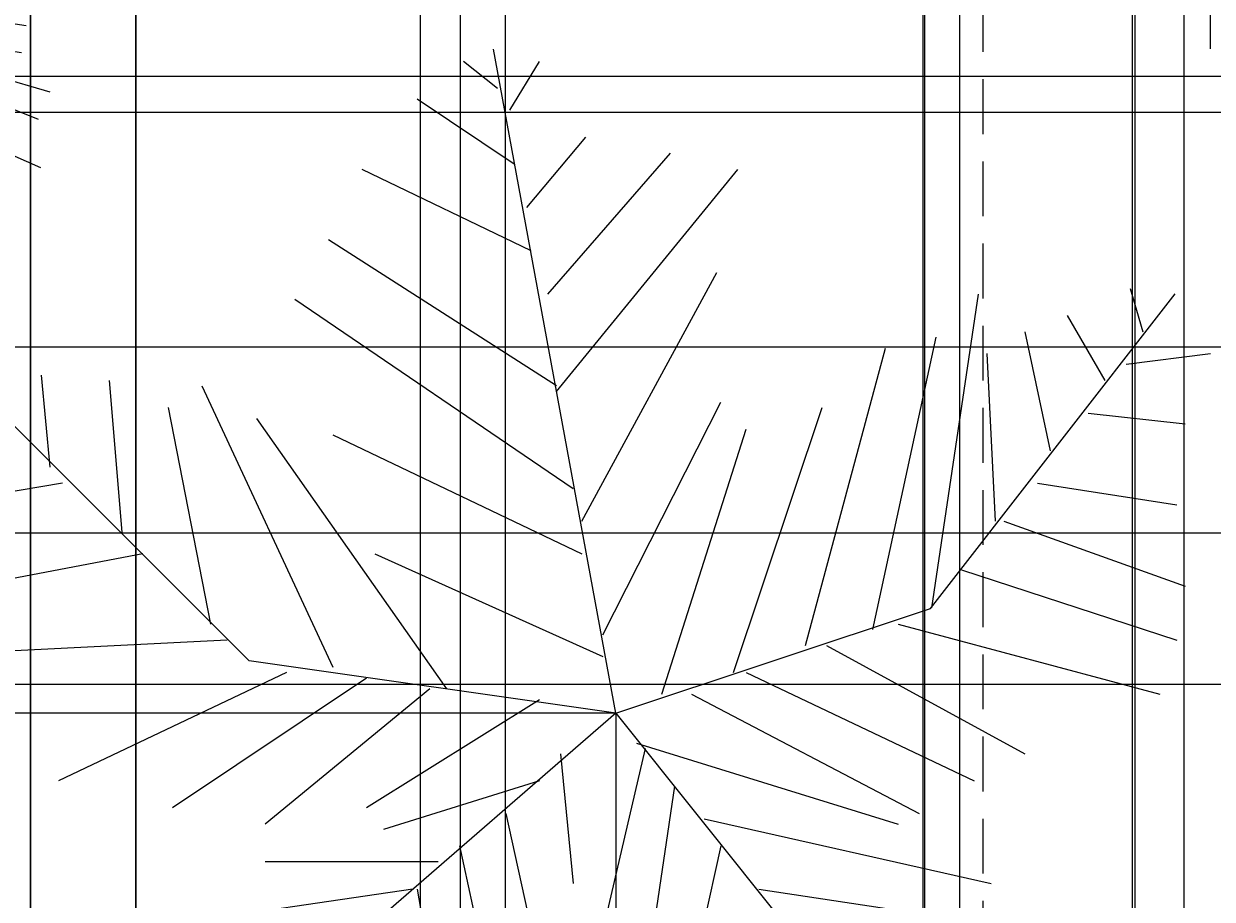
# Model space of a CAD drawing. Units: inches. Extents: x 818 to 1898, y 976 to 2364.
# Tile 13 of 96: x 1071 to 1207, y 1773 to 1873. Entities that reach past the tile are written whole.
import ezdxf

# ---------------------------------------------------------------- set-up
doc = ezdxf.new("R2010")
doc.units = ezdxf.units.IN
doc.header["$LTSCALE"] = 5
doc.header["$MEASUREMENT"] = 0
doc.linetypes.add('HIDDEN', pattern=[0.375, 0.25, -0.125])
for name, color, linetype, lineweight in [('A-ANNO-DIMS', 2, 'Continuous', 18), ('A-FLOR-OVHD', 8, 'HIDDEN', 13), ('L-PLNT-BEDS', 94, 'Continuous', 18)]:
    doc.layers.add(name, color=color, linetype=linetype, lineweight=lineweight)
doc.layers.add('L-PLNT', color=116, linetype='Continuous', lineweight=13, true_color=0x136734)
doc.styles.get("Standard").update_dxf_attribs({"font": 'arial.ttf'})
doc.dimstyles.get("Standard").update_dxf_attribs({"dimtxt": 0.18, "dimasz": 0.18, "dimexe": 0.18, "dimexo": 0.0625, "dimgap": 0.09, "dimtad": 0, "dimtih": 1, "dimtoh": 1, "dimdec": 4, "dimzin": 0, "dimdsep": 46, "dimtxsty": 'Standard', "dimcen": 0.09, "dimadec": 0, "dimazin": 0, "dimtfac": 1, "dimtdec": 4, "dimtofl": 0, "dimtmove": 0, "dimatfit": 3, "dimfxl": 1, "dimtolj": 1, "dimtzin": 0, "dimarcsym": 0})

# ---------------------------------------------------------------- blocks, each defined once
blk = doc.blocks.new('PALM-BORDER')
for p, q in [((41.53, 39.05), (33.72, 81.45)), ((33.95, 78.95), (31.8, 80.68)), ((34.76, 77.57), (36.65, 80.68)), ((35.03, 74.11), (28.83, 78.26)), ((35.84, 71.35), (39.61, 75.84)), ((37.18, 65.82), (45, 74.8)), ((36.11, 68.59), (25.33, 73.77)), ((37.72, 59.6), (49.31, 73.77)), ((37.72, 59.95), (23.17, 69.28)), ((39.34, 51.31), (47.96, 67.2)), ((38.8, 53.39), (21.02, 65.48)), ((61.61, 45.75), (77.23, 65.83)), ((61.71, 45.79), (64.67, 65.82)), ((74.37, 66.17), (75.18, 63.4)), ((70.33, 64.44), (72.75, 60.3)), ((53.62, 43.37), (58.74, 62.37)), ((57.93, 44.41), (61.97, 63.06)), ((67.63, 63.4), (69.25, 55.81)), ((65.21, 62.02), (65.75, 51.31)), ((74.1, 61.33), (79.49, 62.02)), ((5.39, 54.77), (4.85, 60.64)), ((9.16, 60.3), (9.97, 50.62)), ((15.09, 59.95), (23.44, 41.99)), ((12.93, 58.57), (15.63, 44.75)), ((40.69, 44.06), (48.23, 58.91)), ((49.04, 41.64), (54.7, 58.57)), ((18.1, 42.4), (2.48, 58.02)), ((30.72, 40.61), (18.59, 57.88)), ((44.46, 40.26), (49.85, 57.19)), ((71.68, 58.22), (77.87, 57.53)), ((23.44, 56.84), (39.34, 49.24)), ((6.2, 53.73), (0, 52.7)), ((68.44, 53.73), (77.33, 52.35)), ((66.29, 51.31), (77.87, 47.17)), ((11.32, 49.24), (0.54, 47.17)), ((26.14, 49.24), (40.69, 42.68)), ((63.59, 48.21), (77.33, 43.71)), ((41.53, 39.05), (61.61, 45.75)), ((59.55, 44.75), (76.26, 40.26)), ((16.71, 43.71), (2.69, 43.02)), ((41.53, 39.05), (18.1, 42.4)), ((54.97, 43.37), (67.63, 36.46)), ((20.48, 41.64), (5.93, 34.73)), ((25.6, 41.3), (13.2, 33.01)), ((49.85, 41.64), (64.4, 34.73)), ((29.64, 40.61), (19.13, 31.97)), ((36.65, 39.91), (25.6, 33.01)), ((46.35, 40.26), (60.9, 32.66)), ((41.53, 39.05), (24.79, 24.55)), ((41.53, 39.05), (54.92, 22.32)), ((43.38, 36.81), (40.42, 24.02)), ((42.84, 37.15), (59.55, 31.97)), ((37.99, 36.46), (38.8, 28.17)), ((36.65, 34.73), (26.68, 31.62)), ((45.27, 34.39), (43.11, 19.88)), ((34.49, 32.66), (36.92, 21.61)), ((47.15, 32.32), (65.48, 28.17)), ((31.53, 30.59), (35.03, 14.7)), ((48.23, 30.59), (44.19, 12.28)), ((30.18, 29.55), (19.13, 29.55)), ((28.56, 27.82), (9.7, 25.06)), ((28.83, 27.82), (32.07, 9.17)), ((50.66, 27.82), (68.98, 25.06)), ((52, 26.44), (46.35, 9.17)), ((24.79, 24.55), (13.63, 5.58)), ((26.14, 25.41), (28.29, 6.06)), ((53.62, 24.37), (68.44, 21.95)), ((23.44, 22.99), (9.97, 22.64)), ((54.97, 22.3), (47.69, 5.02)), ((54.92, 22.32), (61.61, 0)), ((55.24, 22.3), (71.68, 17.46)), ((22.9, 21.26), (24.52, 5.37)), ((21.56, 19.53), (11.59, 19.88)), ((55.78, 20.22), (70.33, 14.35)), ((20.48, 17.46), (9.7, 15.73)), ((56.59, 16.42), (53.35, 5.72)), ((19.94, 16.08), (20.75, 6.41)), ((18.59, 13.66), (9.97, 12.62)), ((57.39, 14.7), (70.6, 8.83)), ((17.24, 11.59), (17.78, 6.06)), ((58.47, 10.9), (56.05, 2.95)), ((15.9, 9.52), (11.05, 7.44)), ((58.47, 10.55), (67.09, 5.72)), ((59.82, 6.75), (64.4, 3.64)), ((59.82, 5.02), (58.74, 1.22)), ((61.44, 1.92), (62.51, 1.22))]:
    blk.add_line(p, q)
blk = doc.blocks.new('PALM-DECK')
for p, q in [((74.19, 69.77), (60.24, 145.52)), ((60.66, 141.05), (56.81, 144.14)), ((62.1, 138.58), (65.47, 144.14)), ((62.58, 132.41), (51.51, 139.82)), ((64.03, 127.47), (70.77, 135.5)), ((66.43, 117.6), (80.4, 133.65)), ((64.51, 122.54), (45.25, 131.79)), ((67.4, 106.49), (88.1, 131.79)), ((67.4, 107.11), (41.4, 123.77)), ((70.29, 91.68), (85.69, 120.07)), ((132.87, 118.22), (134.31, 113.28)), ((69.32, 95.38), (37.55, 116.98)), ((110.08, 81.73), (137.98, 117.61)), ((110.24, 81.8), (115.54, 117.6)), ((125.65, 115.13), (129.98, 107.72)), ((103.5, 79.33), (110.72, 112.66)), ((120.83, 113.28), (123.72, 99.7)), ((95.8, 77.48), (104.95, 111.43)), ((116.5, 110.81), (117.47, 91.68)), ((132.39, 109.58), (142.02, 110.81)), ((9.63, 97.85), (8.67, 108.34)), ((16.37, 107.72), (17.81, 90.44)), ((26.96, 107.11), (41.88, 75.01)), ((23.11, 104.64), (27.92, 79.95)), ((72.69, 78.72), (86.17, 105.26)), ((87.62, 74.4), (97.73, 104.64)), ((32.33, 75.75), (4.43, 103.66)), ((54.88, 72.55), (33.22, 103.4)), ((128.06, 104.02), (139.13, 102.79)), ((79.43, 71.93), (89.06, 102.17)), ((41.88, 101.55), (70.29, 87.97)), ((11.07, 96), (0, 94.15)), ((122.28, 96), (138.16, 93.53)), ((118.43, 91.68), (139.13, 84.27)), ((20.22, 87.97), (0.96, 84.27)), ((46.7, 87.97), (72.69, 76.25)), ((113.61, 86.12), (138.16, 78.1)), ((74.19, 69.77), (110.08, 81.73)), ((106.39, 79.95), (136.24, 71.93)), ((29.85, 78.1), (4.81, 76.87)), ((98.21, 77.48), (120.83, 65.14)), ((74.19, 69.77), (32.33, 75.75)), ((36.59, 74.4), (10.59, 62.05)), ((45.73, 73.78), (23.59, 58.97)), ((89.06, 74.4), (115.06, 62.05)), ((52.96, 72.55), (34.18, 57.12)), ((82.8, 71.93), (108.8, 58.35)), ((65.47, 71.31), (45.73, 58.97)), ((74.19, 69.77), (44.29, 43.85)), ((74.19, 69.77), (98.11, 39.87)), ((67.88, 65.14), (69.32, 50.33)), ((77.51, 65.76), (72.21, 42.92)), ((76.54, 66.37), (106.39, 57.12)), ((65.47, 62.05), (47.66, 56.5)), ((80.88, 61.44), (77.03, 35.52)), ((61.62, 58.35), (65.95, 38.6)), ((84.25, 57.73), (116.98, 50.33)), ((56.33, 54.65), (62.58, 26.26)), ((86.17, 54.65), (78.95, 21.94)), ((53.92, 52.8), (34.18, 52.8)), ((51.03, 49.71), (17.33, 44.77)), ((51.51, 49.71), (57.29, 16.38)), ((90.51, 49.71), (123.24, 44.77))]:
    blk.add_line(p, q)
blk = doc.blocks.new('*D29')
at = {"layer": 'A-ANNO-DIMS', "color": 0, "lineweight": -2, "ltscale": 5, "transparency": 16777216}
for p, q in [((1064.31, 1870.24), (1064.31, 1892.19)), ((1064.49, 1892.01), (1134.73, 1892.01)), ((1206.15, 1892.01), (1135.91, 1892.01)), ((1206.33, 1870.24), (1206.33, 1892.19))]:
    blk.add_line(p, q, dxfattribs=at)
at = {"layer": 'A-ANNO-DIMS', "color": 0, "ltscale": 5, "transparency": 16777216}
for points in [[(1064.49, 1892.04), (1064.49, 1891.98), (1064.31, 1892.01)], [(1206.15, 1892.04), (1206.15, 1891.98), (1206.33, 1892.01)]]:
    blk.add_solid(points, dxfattribs=at)
at = {"layer": 'Defpoints', "color": 0, "ltscale": 5, "transparency": 16777216}
for p in [(1206.33, 1892.01), (1064.31, 1870.18), (1206.33, 1870.18)]:
    blk.add_point(p, dxfattribs=at)
at = {"layer": 'A-ANNO-DIMS', "color": 0, "ltscale": 5, "transparency": 16777216, "insert": (1135.32, 1892.01), "char_height": 0.18, "attachment_point": 5}
blk.add_mtext('\\A1;142 TYP.', dxfattribs=at)
blk = doc.blocks.new('*D59')
at = {"layer": 'A-ANNO-DIMS', "color": 0, "lineweight": -2, "ltscale": 5, "transparency": 16777216}
for p, q in [((1251.64, 2300.39), (818.03, 2300.39)), ((818.21, 2300.21), (818.21, 1669.95)), ((818.21, 1039.32), (818.21, 1669.59)), ((896.05, 1039.14), (818.03, 1039.14))]:
    blk.add_line(p, q, dxfattribs=at)
at = {"layer": 'A-ANNO-DIMS', "color": 0, "ltscale": 5, "transparency": 16777216}
for points in [[(818.18, 2300.21), (818.24, 2300.21), (818.21, 2300.39)], [(818.18, 1039.32), (818.24, 1039.32), (818.21, 1039.14)]]:
    blk.add_solid(points, dxfattribs=at)
at = {"layer": 'Defpoints', "color": 0, "ltscale": 5, "transparency": 16777216}
for p in [(818.21, 2300.39), (1251.71, 2300.39), (896.11, 1039.14)]:
    blk.add_point(p, dxfattribs=at)
at = {"layer": 'A-ANNO-DIMS', "color": 0, "ltscale": 5, "transparency": 16777216, "insert": (818.21, 1669.77), "char_height": 0.18, "attachment_point": 5}
blk.add_mtext('\\A1;1261.2', dxfattribs=at)
blk = doc.blocks.new('*D61')
at = {"layer": 'A-ANNO-DIMS', "color": 0, "lineweight": -2, "ltscale": 5, "transparency": 16777216}
for p, q in [((1071.73, 1203.03), (1071.73, 2363.87)), ((1071.91, 2363.69), (1250.94, 2363.69)), ((1430.55, 2363.69), (1251.51, 2363.69)), ((1430.73, 1203.03), (1430.73, 2363.87))]:
    blk.add_line(p, q, dxfattribs=at)
at = {"layer": 'A-ANNO-DIMS', "color": 0, "ltscale": 5, "transparency": 16777216}
for points in [[(1071.91, 2363.72), (1071.91, 2363.66), (1071.73, 2363.69)], [(1430.55, 2363.72), (1430.55, 2363.66), (1430.73, 2363.69)]]:
    blk.add_solid(points, dxfattribs=at)
at = {"layer": 'Defpoints', "color": 0, "ltscale": 5, "transparency": 16777216}
for p in [(1430.73, 2363.69), (1071.73, 1202.96), (1430.73, 1202.96)]:
    blk.add_point(p, dxfattribs=at)
at = {"layer": 'A-ANNO-DIMS', "color": 0, "ltscale": 5, "transparency": 16777216, "insert": (1251.23, 2363.69), "char_height": 0.18, "attachment_point": 5}
blk.add_mtext('\\A1;359', dxfattribs=at)
blk = doc.blocks.new('*D64')
at = {"layer": 'A-ANNO-DIMS', "color": 0, "lineweight": -2, "ltscale": 5, "transparency": 16777216}
for p, q in [((1197.73, 1501.14), (1197.73, 2363.87)), ((1197.91, 2363.69), (1313.93, 2363.69)), ((1430.55, 2363.69), (1314.52, 2363.69)), ((1430.73, 1501.14), (1430.73, 2363.87))]:
    blk.add_line(p, q, dxfattribs=at)
at = {"layer": 'A-ANNO-DIMS', "color": 0, "ltscale": 5, "transparency": 16777216}
for points in [[(1197.91, 2363.72), (1197.91, 2363.66), (1197.73, 2363.69)], [(1430.55, 2363.72), (1430.55, 2363.66), (1430.73, 2363.69)]]:
    blk.add_solid(points, dxfattribs=at)
at = {"layer": 'Defpoints', "color": 0, "ltscale": 5, "transparency": 16777216}
for p in [(1430.73, 2363.69), (1197.73, 1501.08), (1430.73, 1501.08)]:
    blk.add_point(p, dxfattribs=at)
at = {"layer": 'A-ANNO-DIMS', "color": 0, "ltscale": 5, "transparency": 16777216, "insert": (1314.23, 2363.69), "char_height": 0.18, "attachment_point": 5}
blk.add_mtext('\\A1;233', dxfattribs=at)
blk = doc.blocks.new('*D79')
at = {"layer": 'A-ANNO-DIMS', "color": 0, "lineweight": -2, "ltscale": 5, "transparency": 16777216}
for p, q in [((992.73, 1203.03), (992.73, 2363.87)), ((992.91, 2363.69), (1032.01, 2363.69)), ((1071.55, 2363.69), (1032.44, 2363.69)), ((1071.73, 1203.03), (1071.73, 2363.87))]:
    blk.add_line(p, q, dxfattribs=at)
at = {"layer": 'A-ANNO-DIMS', "color": 0, "ltscale": 5, "transparency": 16777216}
for points in [[(992.91, 2363.72), (992.91, 2363.66), (992.73, 2363.69)], [(1071.55, 2363.72), (1071.55, 2363.66), (1071.73, 2363.69)]]:
    blk.add_solid(points, dxfattribs=at)
at = {"layer": 'Defpoints', "color": 0, "ltscale": 5, "transparency": 16777216}
for p in [(1071.73, 2363.69), (992.73, 1202.96), (1071.73, 1202.96)]:
    blk.add_point(p, dxfattribs=at)
at = {"layer": 'A-ANNO-DIMS', "color": 0, "ltscale": 5, "transparency": 16777216, "insert": (1032.23, 2363.69), "char_height": 0.18, "attachment_point": 5}
blk.add_mtext('\\A1;79', dxfattribs=at)
blk = doc.blocks.new('*D82')
at = {"layer": 'A-ANNO-DIMS', "color": 0, "lineweight": -2, "ltscale": 5, "transparency": 16777216}
for p, q in [((1083.73, 1501.14), (1083.73, 2363.87)), ((1083.91, 2363.69), (1140.45, 2363.69)), ((1197.55, 2363.69), (1141.01, 2363.69)), ((1197.73, 1501.14), (1197.73, 2363.87))]:
    blk.add_line(p, q, dxfattribs=at)
at = {"layer": 'A-ANNO-DIMS', "color": 0, "ltscale": 5, "transparency": 16777216}
for points in [[(1083.91, 2363.72), (1083.91, 2363.66), (1083.73, 2363.69)], [(1197.55, 2363.72), (1197.55, 2363.66), (1197.73, 2363.69)]]:
    blk.add_solid(points, dxfattribs=at)
at = {"layer": 'Defpoints', "color": 0, "ltscale": 5, "transparency": 16777216}
for p in [(1197.73, 2363.69), (1083.73, 1501.08), (1197.73, 1501.08)]:
    blk.add_point(p, dxfattribs=at)
at = {"layer": 'A-ANNO-DIMS', "color": 0, "ltscale": 5, "transparency": 16777216, "insert": (1140.73, 2363.69), "char_height": 0.18, "attachment_point": 5}
blk.add_mtext('\\A1;114', dxfattribs=at)
blk = doc.blocks.new('*D83')
at = {"layer": 'A-ANNO-DIMS', "color": 0, "lineweight": -2, "ltscale": 5, "transparency": 16777216}
for p, q in [((1197.73, 1700.14), (1197.73, 2363.87)), ((1197.91, 2363.69), (1228.02, 2363.69)), ((1258.55, 2363.69), (1228.43, 2363.69)), ((1258.73, 1700.14), (1258.73, 2363.87))]:
    blk.add_line(p, q, dxfattribs=at)
at = {"layer": 'A-ANNO-DIMS', "color": 0, "ltscale": 5, "transparency": 16777216}
for points in [[(1197.91, 2363.72), (1197.91, 2363.66), (1197.73, 2363.69)], [(1258.55, 2363.72), (1258.55, 2363.66), (1258.73, 2363.69)]]:
    blk.add_solid(points, dxfattribs=at)
at = {"layer": 'Defpoints', "color": 0, "ltscale": 5, "transparency": 16777216}
for p in [(1258.73, 2363.69), (1197.73, 1700.08), (1258.73, 1700.08)]:
    blk.add_point(p, dxfattribs=at)
at = {"layer": 'A-ANNO-DIMS', "color": 0, "ltscale": 5, "transparency": 16777216, "insert": (1228.23, 2363.69), "char_height": 0.18, "attachment_point": 5}
blk.add_mtext('\\A1;61', dxfattribs=at)
blk = doc.blocks.new('*D93')
at = {"layer": 'A-ANNO-DIMS', "color": 0, "lineweight": -2, "ltscale": 5, "transparency": 16777216}
for p, q in [((1068.34, 1071.12), (1068.34, 2363.87)), ((1068.52, 2363.69), (1094.16, 2363.69)), ((1120.58, 2363.69), (1094.94, 2363.69)), ((1120.76, 1071.12), (1120.76, 2363.87))]:
    blk.add_line(p, q, dxfattribs=at)
at = {"layer": 'A-ANNO-DIMS', "color": 0, "ltscale": 5, "transparency": 16777216}
for points in [[(1068.52, 2363.72), (1068.52, 2363.66), (1068.34, 2363.69)], [(1120.58, 2363.72), (1120.58, 2363.66), (1120.76, 2363.69)]]:
    blk.add_solid(points, dxfattribs=at)
at = {"layer": 'Defpoints', "color": 0, "ltscale": 5, "transparency": 16777216}
for p in [(1120.76, 2363.69), (1068.34, 1071.06), (1120.76, 1071.06)]:
    blk.add_point(p, dxfattribs=at)
at = {"layer": 'A-ANNO-DIMS', "color": 0, "ltscale": 5, "transparency": 16777216, "insert": (1094.55, 2363.69), "char_height": 0.18, "attachment_point": 5}
blk.add_mtext('\\A1;52.42', dxfattribs=at)
blk = doc.blocks.new('*D94')
at = {"layer": 'A-ANNO-DIMS', "color": 0, "lineweight": -2, "ltscale": 5, "transparency": 16777216}
for p, q in [((1120.76, 1071.12), (1120.76, 2363.87)), ((1120.94, 2363.69), (1146.76, 2363.69)), ((1173.36, 2363.69), (1147.55, 2363.69)), ((1173.54, 1071.12), (1173.54, 2363.87))]:
    blk.add_line(p, q, dxfattribs=at)
at = {"layer": 'A-ANNO-DIMS', "color": 0, "ltscale": 5, "transparency": 16777216}
for points in [[(1120.94, 2363.72), (1120.94, 2363.66), (1120.76, 2363.69)], [(1173.36, 2363.72), (1173.36, 2363.66), (1173.54, 2363.69)]]:
    blk.add_solid(points, dxfattribs=at)
at = {"layer": 'Defpoints', "color": 0, "ltscale": 5, "transparency": 16777216}
for p in [(1173.54, 2363.69), (1120.76, 1071.06), (1173.54, 1071.06)]:
    blk.add_point(p, dxfattribs=at)
at = {"layer": 'A-ANNO-DIMS', "color": 0, "ltscale": 5, "transparency": 16777216, "insert": (1147.15, 2363.69), "char_height": 0.18, "attachment_point": 5}
blk.add_mtext('\\A1;52.78', dxfattribs=at)
blk = doc.blocks.new('*D95')
at = {"layer": 'A-ANNO-DIMS', "color": 0, "lineweight": -2, "ltscale": 5, "transparency": 16777216}
for p, q in [((1173.54, 1071.12), (1173.54, 2363.87)), ((1173.72, 2363.69), (1201.29, 2363.69)), ((1229.47, 2363.69), (1201.9, 2363.69)), ((1229.65, 1071.12), (1229.65, 2363.87))]:
    blk.add_line(p, q, dxfattribs=at)
at = {"layer": 'A-ANNO-DIMS', "color": 0, "ltscale": 5, "transparency": 16777216}
for points in [[(1173.72, 2363.72), (1173.72, 2363.66), (1173.54, 2363.69)], [(1229.47, 2363.72), (1229.47, 2363.66), (1229.65, 2363.69)]]:
    blk.add_solid(points, dxfattribs=at)
at = {"layer": 'Defpoints', "color": 0, "ltscale": 5, "transparency": 16777216}
for p in [(1229.65, 2363.69), (1173.54, 1071.06), (1229.65, 1071.06)]:
    blk.add_point(p, dxfattribs=at)
at = {"layer": 'A-ANNO-DIMS', "color": 0, "ltscale": 5, "transparency": 16777216, "insert": (1201.59, 2363.69), "char_height": 0.18, "attachment_point": 5}
blk.add_mtext('\\A1;56.1', dxfattribs=at)
blk = doc.blocks.new('*D109')
at = {"layer": 'A-ANNO-DIMS', "color": 0, "lineweight": -2, "ltscale": 5, "transparency": 16777216}
for p, q in [((1125.92, 1410.12), (1125.92, 2363.87)), ((1126.1, 2363.69), (1164.25, 2363.69)), ((1203.15, 2363.69), (1165, 2363.69)), ((1203.33, 1409.91), (1203.33, 2363.87))]:
    blk.add_line(p, q, dxfattribs=at)
at = {"layer": 'A-ANNO-DIMS', "color": 0, "ltscale": 5, "transparency": 16777216}
for points in [[(1126.1, 2363.72), (1126.1, 2363.66), (1125.92, 2363.69)], [(1203.15, 2363.72), (1203.15, 2363.66), (1203.33, 2363.69)]]:
    blk.add_solid(points, dxfattribs=at)
at = {"layer": 'Defpoints', "color": 0, "ltscale": 5, "transparency": 16777216}
for p in [(1203.33, 2363.69), (1125.92, 1410.05), (1203.33, 1409.85)]:
    blk.add_point(p, dxfattribs=at)
at = {"layer": 'A-ANNO-DIMS', "color": 0, "ltscale": 5, "transparency": 16777216, "insert": (1164.62, 2363.69), "char_height": 0.18, "attachment_point": 5}
blk.add_mtext('\\A1;77.41', dxfattribs=at)
blk = doc.blocks.new('*D120')
at = {"layer": 'A-ANNO-DIMS', "color": 0, "lineweight": -2, "ltscale": 5, "transparency": 16777216}
for p, q in [((1766.29, 1797.72), (818.03, 1797.72)), ((818.21, 1797.54), (818.21, 1757.53)), ((818.21, 1717.17), (818.21, 1757.17)), ((1766.29, 1716.99), (818.03, 1716.99))]:
    blk.add_line(p, q, dxfattribs=at)
at = {"layer": 'A-ANNO-DIMS', "color": 0, "ltscale": 5, "transparency": 16777216}
for points in [[(818.18, 1797.54), (818.24, 1797.54), (818.21, 1797.72)], [(818.18, 1717.17), (818.24, 1717.17), (818.21, 1716.99)]]:
    blk.add_solid(points, dxfattribs=at)
at = {"layer": 'Defpoints', "color": 0, "ltscale": 5, "transparency": 16777216}
for p in [(818.21, 1797.72), (1766.35, 1797.72), (1766.35, 1716.99)]:
    blk.add_point(p, dxfattribs=at)
at = {"layer": 'A-ANNO-DIMS', "color": 0, "ltscale": 5, "transparency": 16777216, "insert": (818.21, 1757.35), "char_height": 0.18, "attachment_point": 5}
blk.add_mtext('\\A1;80.73', dxfattribs=at)
blk = doc.blocks.new('*D121')
at = {"layer": 'A-ANNO-DIMS', "color": 0, "lineweight": -2, "ltscale": 5, "transparency": 16777216}
for p, q in [((1766.29, 1884.2), (818.03, 1884.2)), ((818.21, 1884.02), (818.21, 1841.14)), ((818.21, 1797.9), (818.21, 1840.78)), ((1766.29, 1797.72), (818.03, 1797.72))]:
    blk.add_line(p, q, dxfattribs=at)
at = {"layer": 'A-ANNO-DIMS', "color": 0, "ltscale": 5, "transparency": 16777216}
for points in [[(818.18, 1884.02), (818.24, 1884.02), (818.21, 1884.2)], [(818.18, 1797.9), (818.24, 1797.9), (818.21, 1797.72)]]:
    blk.add_solid(points, dxfattribs=at)
at = {"layer": 'Defpoints', "color": 0, "ltscale": 5, "transparency": 16777216}
for p in [(818.21, 1884.2), (1766.35, 1884.2), (1766.35, 1797.72)]:
    blk.add_point(p, dxfattribs=at)
at = {"layer": 'A-ANNO-DIMS', "color": 0, "ltscale": 5, "transparency": 16777216, "insert": (818.21, 1840.96), "char_height": 0.18, "attachment_point": 5}
blk.add_mtext('\\A1;86.49', dxfattribs=at)
blk = doc.blocks.new('*D122')
at = {"layer": 'A-ANNO-DIMS', "color": 0, "lineweight": -2, "ltscale": 5, "transparency": 16777216}
for p, q in [((1138.5, 1794.37), (1138.5, 975.66)), ((1071.73, 1688.02), (1071.73, 975.66)), ((1071.91, 975.84), (1104.72, 975.84)), ((1138.32, 975.84), (1105.51, 975.84))]:
    blk.add_line(p, q, dxfattribs=at)
at = {"layer": 'A-ANNO-DIMS', "color": 0, "ltscale": 5, "transparency": 16777216}
for points in [[(1071.91, 975.87), (1071.91, 975.81), (1071.73, 975.84)], [(1138.32, 975.87), (1138.32, 975.81), (1138.5, 975.84)]]:
    blk.add_solid(points, dxfattribs=at)
at = {"layer": 'Defpoints', "color": 0, "ltscale": 5, "transparency": 16777216}
for p in [(1138.5, 1794.43), (1071.73, 1688.08), (1138.5, 975.84)]:
    blk.add_point(p, dxfattribs=at)
at = {"layer": 'A-ANNO-DIMS', "color": 0, "ltscale": 5, "transparency": 16777216, "insert": (1105.11, 975.84), "char_height": 0.18, "attachment_point": 5}
blk.add_mtext('\\A1;66.78', dxfattribs=at)
blk = doc.blocks.new('*D124')
at = {"layer": 'A-ANNO-DIMS', "color": 0, "lineweight": -2, "ltscale": 5, "transparency": 16777216}
for p, q in [((1131.7, 1974.57), (818.03, 1974.57)), ((818.21, 1974.39), (818.21, 1884.68)), ((818.21, 1794.61), (818.21, 1884.32)), ((1138.44, 1794.43), (818.03, 1794.43))]:
    blk.add_line(p, q, dxfattribs=at)
at = {"layer": 'A-ANNO-DIMS', "color": 0, "ltscale": 5, "transparency": 16777216}
for points in [[(818.18, 1974.39), (818.24, 1974.39), (818.21, 1974.57)], [(818.18, 1794.61), (818.24, 1794.61), (818.21, 1794.43)]]:
    blk.add_solid(points, dxfattribs=at)
at = {"layer": 'Defpoints', "color": 0, "ltscale": 5, "transparency": 16777216}
for p in [(818.21, 1974.57), (1131.77, 1974.57), (1138.5, 1794.43)]:
    blk.add_point(p, dxfattribs=at)
at = {"layer": 'A-ANNO-DIMS', "color": 0, "ltscale": 5, "transparency": 16777216, "insert": (818.21, 1884.5), "char_height": 0.18, "attachment_point": 5}
blk.add_mtext('\\A1;180.14', dxfattribs=at)
blk = doc.blocks.new('*D126')
at = {"layer": 'A-ANNO-DIMS', "color": 0, "lineweight": -2, "ltscale": 5, "transparency": 16777216}
for p, q in [((1035.38, 1252.09), (1035.38, 2363.87)), ((1035.56, 2363.69), (1075.41, 2363.69)), ((1116.01, 2363.69), (1076.16, 2363.69)), ((1116.19, 1236.03), (1116.19, 2363.87))]:
    blk.add_line(p, q, dxfattribs=at)
at = {"layer": 'A-ANNO-DIMS', "color": 0, "ltscale": 5, "transparency": 16777216}
for points in [[(1035.56, 2363.72), (1035.56, 2363.66), (1035.38, 2363.69)], [(1116.01, 2363.72), (1116.01, 2363.66), (1116.19, 2363.69)]]:
    blk.add_solid(points, dxfattribs=at)
at = {"layer": 'Defpoints', "color": 0, "ltscale": 5, "transparency": 16777216}
for p in [(1035.38, 2363.69), (1035.38, 1252.02), (1116.19, 1235.96)]:
    blk.add_point(p, dxfattribs=at)
at = {"layer": 'A-ANNO-DIMS', "color": 0, "ltscale": 5, "transparency": 16777216, "insert": (1075.78, 2363.69), "char_height": 0.18, "attachment_point": 5}
blk.add_mtext('\\A1;80.81', dxfattribs=at)
blk = doc.blocks.new('*D145')
at = {"layer": 'A-ANNO-DIMS', "color": 0, "lineweight": -2, "ltscale": 5, "transparency": 16777216}
for p, q in [((1197.39, 2122.31), (1197.39, 975.66)), ((1232.61, 2122.31), (1232.61, 975.66)), ((1197.57, 975.84), (1214.61, 975.84)), ((1232.43, 975.84), (1215.39, 975.84))]:
    blk.add_line(p, q, dxfattribs=at)
at = {"layer": 'A-ANNO-DIMS', "color": 0, "ltscale": 5, "transparency": 16777216}
for points in [[(1197.57, 975.87), (1197.57, 975.81), (1197.39, 975.84)], [(1232.43, 975.87), (1232.43, 975.81), (1232.61, 975.84)]]:
    blk.add_solid(points, dxfattribs=at)
at = {"layer": 'Defpoints', "color": 0, "ltscale": 5, "transparency": 16777216}
for p in [(1197.39, 2122.38), (1232.61, 2122.38), (1232.61, 975.84)]:
    blk.add_point(p, dxfattribs=at)
at = {"layer": 'A-ANNO-DIMS', "color": 0, "ltscale": 5, "transparency": 16777216, "insert": (1215, 975.84), "char_height": 0.18, "attachment_point": 5}
blk.add_mtext('\\A1;35.22', dxfattribs=at)
blk = doc.blocks.new('*D158')
at = {"layer": 'A-ANNO-DIMS', "color": 0, "lineweight": -2, "ltscale": 5, "transparency": 16777216}
for p, q in [((1173.73, 1590.82), (1173.73, 2363.87)), ((1173.91, 2363.69), (1175.57, 2363.69)), ((1177.55, 2363.69), (1175.88, 2363.69)), ((1177.73, 1586.82), (1177.73, 2363.87))]:
    blk.add_line(p, q, dxfattribs=at)
at = {"layer": 'A-ANNO-DIMS', "color": 0, "ltscale": 5, "transparency": 16777216}
for points in [[(1173.91, 2363.72), (1173.91, 2363.66), (1173.73, 2363.69)], [(1177.55, 2363.72), (1177.55, 2363.66), (1177.73, 2363.69)]]:
    blk.add_solid(points, dxfattribs=at)
at = {"layer": 'Defpoints', "color": 0, "ltscale": 5, "transparency": 16777216}
for p in [(1177.73, 2363.69), (1173.73, 1590.76), (1177.73, 1586.76)]:
    blk.add_point(p, dxfattribs=at)
at = {"layer": 'A-ANNO-DIMS', "color": 0, "ltscale": 5, "transparency": 16777216, "insert": (1175.73, 2363.69), "char_height": 0.18, "attachment_point": 5}
blk.add_mtext('\\A1;4', dxfattribs=at)
blk = doc.blocks.new('*D162')
at = {"layer": 'A-ANNO-DIMS', "color": 0, "lineweight": -2, "ltscale": 5, "transparency": 16777216}
for p, q in [((1429.16, 1876.08), (818.03, 1876.08)), ((818.21, 1875.9), (818.21, 1871.76)), ((818.21, 1867.26), (818.21, 1871.4)), ((1429.16, 1867.08), (818.03, 1867.08))]:
    blk.add_line(p, q, dxfattribs=at)
at = {"layer": 'A-ANNO-DIMS', "color": 0, "ltscale": 5, "transparency": 16777216}
for points in [[(818.18, 1875.9), (818.24, 1875.9), (818.21, 1876.08)], [(818.18, 1867.26), (818.24, 1867.26), (818.21, 1867.08)]]:
    blk.add_solid(points, dxfattribs=at)
at = {"layer": 'Defpoints', "color": 0, "ltscale": 5, "transparency": 16777216}
for p in [(1429.23, 1876.08), (818.21, 1867.08), (1429.23, 1867.08)]:
    blk.add_point(p, dxfattribs=at)
at = {"layer": 'A-ANNO-DIMS', "color": 0, "ltscale": 5, "transparency": 16777216, "insert": (818.21, 1871.58), "char_height": 0.18, "attachment_point": 5}
blk.add_mtext('\\A1;9', dxfattribs=at)
blk = doc.blocks.new('*D215')
at = {"layer": 'A-ANNO-DIMS', "color": 0, "lineweight": -2, "ltscale": 5, "transparency": 16777216}
for p, q in [((1590.66, 1876.08), (818.03, 1876.08)), ((818.21, 1875.9), (818.21, 1781.76)), ((818.21, 1687.26), (818.21, 1781.4)), ((1511.66, 1687.08), (818.03, 1687.08))]:
    blk.add_line(p, q, dxfattribs=at)
at = {"layer": 'A-ANNO-DIMS', "color": 0, "ltscale": 5, "transparency": 16777216}
for points in [[(818.18, 1875.9), (818.24, 1875.9), (818.21, 1876.08)], [(818.18, 1687.26), (818.24, 1687.26), (818.21, 1687.08)]]:
    blk.add_solid(points, dxfattribs=at)
at = {"layer": 'Defpoints', "color": 0, "ltscale": 5, "transparency": 16777216}
for p in [(818.21, 1876.08), (1590.73, 1876.08), (1511.73, 1687.08)]:
    blk.add_point(p, dxfattribs=at)
at = {"layer": 'A-ANNO-DIMS', "color": 0, "ltscale": 5, "transparency": 16777216, "insert": (818.21, 1781.58), "char_height": 0.18, "attachment_point": 5}
blk.add_mtext('\\A1;189', dxfattribs=at)
blk = doc.blocks.new('*D227')
at = {"layer": 'A-ANNO-DIMS', "color": 0, "lineweight": -2, "ltscale": 5, "transparency": 16777216}
for p, q in [((1595.66, 1867.08), (818.03, 1867.08)), ((818.21, 1866.9), (818.21, 1851.81)), ((818.21, 1836.36), (818.21, 1851.45)), ((1594.66, 1836.18), (818.03, 1836.18))]:
    blk.add_line(p, q, dxfattribs=at)
at = {"layer": 'A-ANNO-DIMS', "color": 0, "ltscale": 5, "transparency": 16777216}
for points in [[(818.18, 1866.9), (818.24, 1866.9), (818.21, 1867.08)], [(818.18, 1836.36), (818.24, 1836.36), (818.21, 1836.18)]]:
    blk.add_solid(points, dxfattribs=at)
at = {"layer": 'Defpoints', "color": 0, "ltscale": 5, "transparency": 16777216}
for p in [(818.21, 1867.08), (1595.73, 1867.08), (1594.73, 1836.18)]:
    blk.add_point(p, dxfattribs=at)
at = {"layer": 'A-ANNO-DIMS', "color": 0, "ltscale": 5, "transparency": 16777216, "insert": (818.21, 1851.63), "char_height": 0.18, "attachment_point": 5}
blk.add_mtext('\\A1;30.894', dxfattribs=at)
blk = doc.blocks.new('*D247')
at = {"layer": 'A-ANNO-DIMS', "color": 0, "lineweight": -2, "ltscale": 5, "transparency": 16777216}
for p, q in [((1258.66, 1862.97), (818.03, 1862.97)), ((818.21, 1862.79), (818.21, 1839.15)), ((818.21, 1815.15), (818.21, 1838.78)), ((1258.66, 1814.97), (818.03, 1814.97))]:
    blk.add_line(p, q, dxfattribs=at)
at = {"layer": 'A-ANNO-DIMS', "color": 0, "ltscale": 5, "transparency": 16777216}
for points in [[(818.18, 1862.79), (818.24, 1862.79), (818.21, 1862.97)], [(818.18, 1815.15), (818.24, 1815.15), (818.21, 1814.97)]]:
    blk.add_solid(points, dxfattribs=at)
at = {"layer": 'Defpoints', "color": 0, "ltscale": 5, "transparency": 16777216}
for p in [(818.21, 1862.97), (1258.73, 1862.97), (1258.73, 1814.97)]:
    blk.add_point(p, dxfattribs=at)
at = {"layer": 'A-ANNO-DIMS', "color": 0, "ltscale": 5, "transparency": 16777216, "insert": (818.21, 1838.97), "char_height": 0.18, "attachment_point": 5}
blk.add_mtext('\\A1;48', dxfattribs=at)
blk = doc.blocks.new('*D249')
at = {"layer": 'A-ANNO-DIMS', "color": 0, "lineweight": -2, "ltscale": 5, "transparency": 16777216}
for p, q in [((1258.66, 1814.97), (818.03, 1814.97)), ((818.21, 1814.79), (818.21, 1785.33)), ((818.21, 1755.51), (818.21, 1784.97)), ((1258.66, 1755.33), (818.03, 1755.33))]:
    blk.add_line(p, q, dxfattribs=at)
at = {"layer": 'A-ANNO-DIMS', "color": 0, "ltscale": 5, "transparency": 16777216}
for points in [[(818.18, 1814.79), (818.24, 1814.79), (818.21, 1814.97)], [(818.18, 1755.51), (818.24, 1755.51), (818.21, 1755.33)]]:
    blk.add_solid(points, dxfattribs=at)
at = {"layer": 'Defpoints', "color": 0, "ltscale": 5, "transparency": 16777216}
for p in [(818.21, 1814.97), (1258.73, 1814.97), (1258.73, 1755.33)]:
    blk.add_point(p, dxfattribs=at)
at = {"layer": 'A-ANNO-DIMS', "color": 0, "ltscale": 5, "transparency": 16777216, "insert": (818.21, 1785.15), "char_height": 0.18, "attachment_point": 5}
blk.add_mtext('\\A1;59.63', dxfattribs=at)

msp = doc.modelspace()

# ---------------------------------------------------------------- linework, layer by layer
at = {"layer": 'A-FLOR-OVHD', "ltscale": 5}
msp.add_line((1180.349, 1913.6401), (1180.349, 1688.0782), dxfattribs=at)
at = {"layer": 'L-PLNT-BEDS'}
for p, q in [((1071.7251, 2214.9709), (1071.7251, 1202.9642)), ((1083.7251, 2044.0782), (1083.7251, 1211.9642))]:
    msp.add_line(p, q, dxfattribs=at)

# ---------------------------------------------------------------- block references
at = {"layer": 'L-PLNT'}
for name, p in [('PALM-BORDER', (1002.2407, 1847.8507)), ('PALM-DECK', (1064.31, 1724.664))]:
    msp.add_blockref(name, p, dxfattribs=at)

# ---------------------------------------------------------------- dimensions: what is measured, and where the dimension line sits
at = {"layer": 'A-ANNO-DIMS', "ltscale": 5}
for base, p1, p2, override, picture, middle in [((1071.7251, 2363.6929), (992.7251, 1202.9642), (1071.7251, 1202.9642), {"dimdec": 0, "dimlfac": 1, "dimrnd": 0, "dimzin": 0, "dimdsep": 46, "dimlunit": 2}, '*D79', (1032.2251, 2363.6929)), ((1035.3768, 2363.6929), (1116.1882, 1235.9642), (1035.3768, 1252.0242), {"dimdec": 2, "dimlfac": 1, "dimrnd": 0, "dimzin": 0, "dimdsep": 46, "dimlunit": 2}, '*D126', (1075.7825, 2363.6929)), ((1120.7618, 2363.6929), (1068.3377, 1071.0552), (1120.7618, 1071.0552), {"dimdec": 2, "dimlfac": 1, "dimrnd": 0, "dimzin": 0, "dimdsep": 46, "dimlunit": 2}, '*D93', (1094.5497, 2363.6929)), ((1430.7251, 2363.6929), (1071.7251, 1202.9642), (1430.7251, 1202.9642), {"dimdec": 0, "dimlfac": 1, "dimrnd": 0, "dimzin": 0, "dimdsep": 46, "dimlunit": 2}, '*D61', (1251.2251, 2363.6929)), ((1197.7251, 2363.6929), (1083.7251, 1501.0782), (1197.7251, 1501.0782), {"dimdec": 0, "dimlfac": 1, "dimrnd": 0, "dimzin": 0, "dimdsep": 46, "dimlunit": 2}, '*D82', (1140.7251, 2363.6929)), ((1173.5418, 2363.6929), (1120.7618, 1071.0552), (1173.5418, 1071.0552), {"dimdec": 2, "dimlfac": 1, "dimrnd": 0, "dimzin": 0, "dimdsep": 46, "dimlunit": 2}, '*D94', (1147.1518, 2363.6929)), ((1203.3292, 2363.6929), (1125.9172, 1410.0547), (1203.3292, 1409.8484), {"dimdec": 2, "dimlfac": 1, "dimrnd": 0, "dimzin": 0, "dimdsep": 46, "dimlunit": 2}, '*D109', (1164.6232, 2363.6929)), ((1229.6474, 2363.6929), (1173.5418, 1071.0552), (1229.6474, 1071.0552), {"dimdec": 1, "dimlfac": 1, "dimrnd": 0, "dimzin": 0, "dimdsep": 46, "dimlunit": 2}, '*D95', (1201.5946, 2363.6929)), ((1177.7251, 2363.6929), (1173.7251, 1590.7585), (1177.7251, 1586.7585), {"dimdec": 0, "dimlfac": 1, "dimrnd": 0, "dimzin": 0, "dimdsep": 46, "dimlunit": 2}, '*D158', (1175.7251, 2363.6929)), ((1430.7251, 2363.6929), (1197.7251, 1501.0782), (1430.7251, 1501.0782), {"dimdec": 0, "dimlfac": 1, "dimrnd": 0, "dimzin": 0, "dimdsep": 46, "dimlunit": 2}, '*D64', (1314.2251, 2363.6929)), ((1258.7251, 2363.6929), (1197.7251, 1700.0782), (1258.7251, 1700.0782), {"dimdec": 0, "dimlfac": 1, "dimrnd": 0, "dimzin": 0, "dimdsep": 46, "dimlunit": 2}, '*D83', (1228.2251, 2363.6929)), ((1232.6091, 975.8433), (1197.3925, 2122.3767), (1232.6091, 2122.3767), {"dimdec": 2, "dimlfac": 1, "dimrnd": 0, "dimzin": 0, "dimdsep": 46, "dimlunit": 2}, '*D145', (1215.0008, 975.8433)), ((1138.5041, 975.8433), (1071.7251, 1688.0782), (1138.5041, 1794.4325), {"dimdec": 2, "dimlfac": 1, "dimrnd": 0, "dimzin": 0, "dimdsep": 46, "dimlunit": 2}, '*D122', (1105.1146, 975.8433))]:
    dim = msp.add_linear_dim(base=base, p1=p1, p2=p2, dimstyle='Standard', override=override, dxfattribs=at)
    dim.commit()
    dim.dimension.update_dxf_attribs({"geometry": picture, "text_midpoint": middle})
for base, p1, p2, override, picture, middle in [((818.2059, 2300.3929), (896.1138, 1039.1433), (1251.7057, 2300.3929), {"dimdec": 1, "dimlfac": 1, "dimrnd": 0, "dimzin": 0, "dimdsep": 46, "dimlunit": 2}, '*D59', (818.2059, 1669.7681)), ((818.2059, 1974.5735), (1138.5041, 1794.4325), (1131.7651, 1974.5735), {"dimdec": 2, "dimlfac": 1, "dimrnd": 0, "dimzin": 0, "dimdsep": 46, "dimlunit": 2}, '*D124', (818.2059, 1884.503)), ((818.2059, 1884.2031), (1766.3524, 1797.7165), (1766.3524, 1884.2031), {"dimdec": 2, "dimlfac": 1, "dimrnd": 0, "dimzin": 0, "dimdsep": 46, "dimlunit": 2}, '*D121', (818.2059, 1840.9598)), ((818.2059, 1876.0782), (1511.7251, 1687.0782), (1590.7251, 1876.0782), {"dimdec": 0, "dimlfac": 1, "dimrnd": 0, "dimzin": 0, "dimdsep": 46, "dimlunit": 2}, '*D215', (818.2059, 1781.5782)), ((818.2059, 1867.0782), (1429.2251, 1876.0782), (1429.2251, 1867.0782), {"dimdec": 0, "dimlfac": 1, "dimrnd": 0, "dimzin": 0, "dimdsep": 46, "dimlunit": 2}, '*D162', (818.2059, 1871.5782)), ((818.2059, 1867.0782), (1594.7251, 1836.1844), (1595.7251, 1867.0782), {"dimdec": 3, "dimlfac": 1, "dimrnd": 0, "dimzin": 0, "dimdsep": 46, "dimlunit": 2}, '*D227', (818.2059, 1851.6313)), ((818.2059, 1862.9652), (1258.7251, 1814.9652), (1258.7251, 1862.9652), {"dimdec": 0, "dimlfac": 1, "dimrnd": 0, "dimzin": 0, "dimdsep": 46, "dimlunit": 2}, '*D247', (818.2059, 1838.9652)), ((818.2059, 1814.9652), (1258.7251, 1755.3321), (1258.7251, 1814.9652), {"dimdec": 2, "dimlfac": 1, "dimrnd": 0, "dimzin": 0, "dimdsep": 46, "dimlunit": 2}, '*D249', (818.2059, 1785.1486)), ((818.2059, 1797.7165), (1766.3524, 1716.9866), (1766.3524, 1797.7165), {"dimdec": 2, "dimlfac": 1, "dimrnd": 0, "dimzin": 0, "dimdsep": 46, "dimlunit": 2}, '*D120', (818.2059, 1757.3516))]:
    dim = msp.add_linear_dim(base=base, p1=p1, p2=p2, angle=90, dimstyle='Standard', override=override, dxfattribs=at)
    dim.commit()
    dim.dimension.update_dxf_attribs({"geometry": picture, "text_midpoint": middle})
dim = msp.add_linear_dim(base=(1206.3272, 1892.009), p1=(1064.3101, 1870.1814), p2=(1206.3272, 1870.1814), text='<> TYP.', dimstyle='Standard', override={"dimdec": 0, "dimlfac": 1, "dimrnd": 0, "dimzin": 0, "dimdsep": 46, "dimlunit": 2}, dxfattribs=at)
dim.commit()
dim.dimension.update_dxf_attribs({"geometry": '*D29', "text_midpoint": (1135.3187, 1892.009)})

doc.saveas('drawing.dxf')
